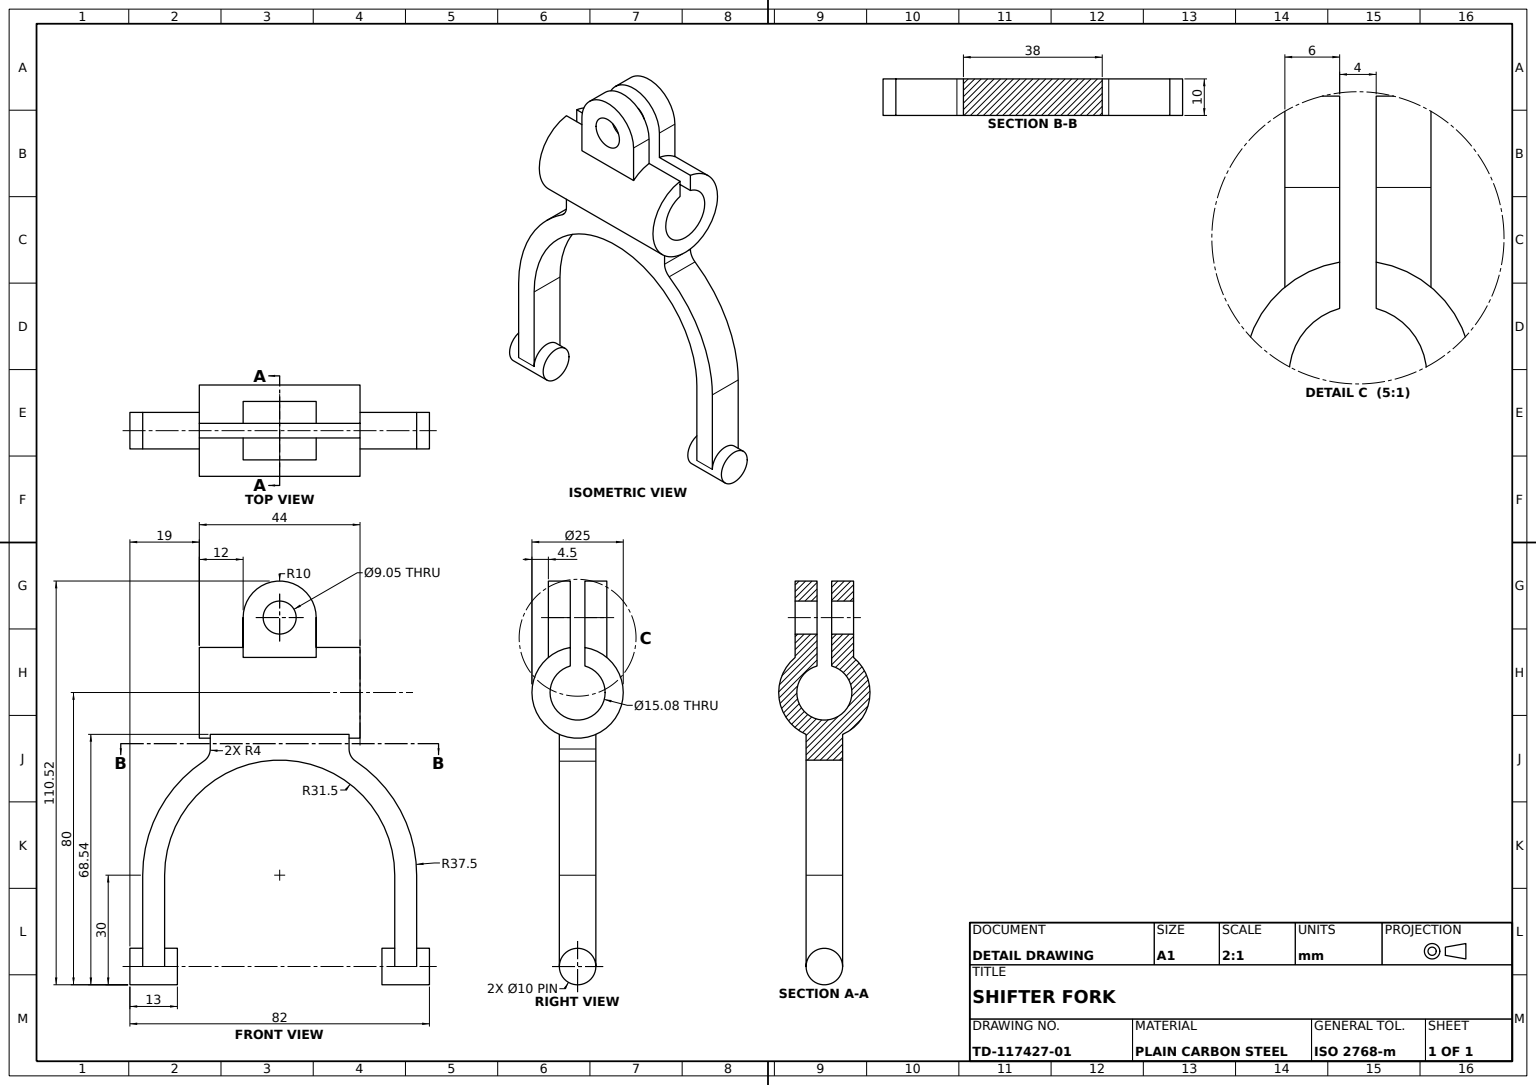
SolidWorks part; units mm, degrees
material "Plain Carbon Steel"
ref_plane "Front Plane" through (0, 0, 0) normal (0, 0, 1) x (1, 0, 0)
ref_plane "Top Plane" through (0, 0, 0) normal (0, 1, 0) x (1, 0, 0)
ref_plane "Right Plane" through (0, 0, 0) normal (1, 0, 0) x (0, 0, -1)
sketch "U-Fork Profile Sketch" plane through (0, 0, 0) normal (0, 0, 1) x (1, 0, 0)
  line L0 (-19, 0) -> (19, 0)
  line L1 (-37.4958, -75) -> (-31.4958, -75)
  line L2 (-37.4958, -75) -> (-37.4958, -50)
  line L3 (-37.4958, -75) -> (-31.4958, -75)
  line L4 (37.5042, -75) -> (31.5042, -75)
  line L5 (37.5042, -50) -> (37.5042, -75)
  line L6 (-31.4958, -75) -> (-31.4958, -50)
  line L7 (31.5042, -50) -> (31.5042, -75)
  line L8 (-19, 0) -> (-19, -17.6721)
  line L9 (19, 0) -> (19, -17.6672)
  line L10 (31.5042, -75) -> (37.5042, -75)
  arc A0 (-31.4958, -50) -> (31.5042, -50) centre (0.0042, -50) cw
  arc A1 (-37.4958, -50) -> (-19, -17.6721) centre (0.0042, -50) cw
  arc A2 (19, -17.6672) -> (37.5042, -50) centre (0.0042, -50) cw
  point P4 (0, 0)
  point P8 (0.0042, -75)
  dimension "D4" = 31.5
  dimension "D1" = 38
  dimension "D2" = 75
  dimension "D3" = 75
  dimension "D5" = 18.4958
  dimension "D6" = 25
extrude "U-Fork Plate" add sketch "U-Fork Profile Sketch" along normal blind 10 contours A2 L9 L0 L8 A1 L2 L1 L6 A0 L7 L4 L5
ref_plane "Plane1" through (0, 0, 0) normal (1, 0, 0) x (0, 0, -1)
sketch "Collar Sketch" plane through (0, 0, 0) normal (1, 0, 0) x (0, 0, -1)
  line L0 (-10, 0) -> (0, 0) construction
  line L4 (-7, 7.2699) -> (-7, 12.339)
  line L5 (-3, 7.2699) -> (-3, 12.339)
  arc A0 (-7, 12.339) -> (-3, 12.339) centre (-5, 0) ccw
  arc A1 (-7, 7.2699) -> (-3, 7.2699) centre (-5, 0) ccw
  point P5 (-5, -12.5)
  point P6 (-5, 12.5)
  point P7 (-3, -12.5)
  point P8 (-3, 12.5)
  point P9 (-7, -12.5)
  point P10 (-7, 12.5)
  dimension "D1" = 25
  dimension "D2" = 15.08
  dimension "D3" = 2
extrude "Split Collar" add sketch "Collar Sketch" along normal mid plane 44
sketch "Collar Bore Sketch" plane through (19, 0, 0) normal (1, 0, 0) x (0, 0, -1)
  line L0 (-10, 0) -> (0, 0) construction
  circle A0 centre (-5, 0) radius 7.54
  dimension "D1" = 15.08
extrude "Collar Bore" cut sketch "Collar Bore Sketch" against normal blind 44
ref_plane "Plane2" through (0, 0, 7) normal (0, 0, 1) x (1, 0, 0)
sketch "Eye Lug Front Sketch" plane through (0, 0, 7) normal (0, 0, 1) x (1, 0, 0)
  line L0 (-10, 5.5162) -> (10, 5.5162)
  line L1 (-10, 5.5162) -> (-10, 20.5162)
  line L2 (10, 5.5162) -> (10, 20.5162)
  arc A0 (-10, 20.5162) -> (10, 20.5162) centre (0, 20.5162) cw
  circle A1 centre (0, 20.5162) radius 4.525
  point P3 (0, 5.5162)
  dimension "D2" = 9.05
  dimension "D3" = 15
  dimension "D1" = 10
  dimension "D4" = 5.5162
extrude "Eye Lug Front" add sketch "Eye Lug Front Sketch" along normal blind 6
ref_plane "Plane3" through (0, 0, 3) normal (0, 0, 1) x (1, 0, 0)
sketch "Eye Lug Rear Sketch" plane through (0, 0, 3) normal (0, 0, 1) x (1, 0, 0)
  line L0 (10, 20.5162) -> (10, 5.5162)
  line L1 (10, 5.5162) -> (-10, 5.5162)
  line L2 (-10, 5.5162) -> (-10, 20.5162)
  line L3 (-10, 20.5162) -> (-10, 12.339) construction
  arc A0 (10, 20.5162) -> (-10, 20.5162) centre (0, 20.5162) ccw construction
  arc A1 (10, 20.5162) -> (-10, 20.5162) centre (0, 20.5162) ccw
  circle A2 centre (0, 20.5162) radius 4.525
  dimension "D1" = 9.05
  dimension "D2" = 15
extrude "Eye Lug Rear" add sketch "Eye Lug Rear Sketch" against normal blind 6
sketch "Eye Hole Sketch" plane through (-10, 0, 0) normal (-1, 0, 0) x (0, 0, 1)
  circle A0 centre (5, 0) radius 7.54
  dimension "D1" = 15.08
extrude "Eye Cross Hole" cut sketch "Eye Hole Sketch" against normal blind 30
ref_plane "Plane4" through (34.5, 0, 0) normal (1, 0, 0) x (0, 0, -1)
sketch "Fork Pin A Sketch" plane through (34.5, 0, 0) normal (1, 0, 0) x (0, 0, -1)
  line L0 (-10, -75) -> (0, -75) construction
  circle A0 centre (-5, -75) radius 5
  dimension "D1" = 10
extrude "Fork Pin A Ø10" add sketch "Fork Pin A Sketch" along normal mid plane 13
ref_plane "Plane5" through (-34.5, 0, 0) normal (1, 0, 0) x (0, 0, -1)
sketch "Fork Pin B Sketch" plane through (-34.5, 0, 0) normal (1, 0, 0) x (0, 0, -1)
  line L0 (-10, -75) -> (0, -75) construction
  circle A0 centre (-5, -75) radius 5
  dimension "D1" = 10
extrude "Fork Pin B Ø10" add sketch "Fork Pin B Sketch" along normal mid plane 13
fillet "Fork Edge Fillet R4 A" radius 4 1 edges at (19, -17.6672, 5)
fillet "Fork Edge Fillet R4 B" radius 4 1 edges at (-19, -17.6721, 5)
